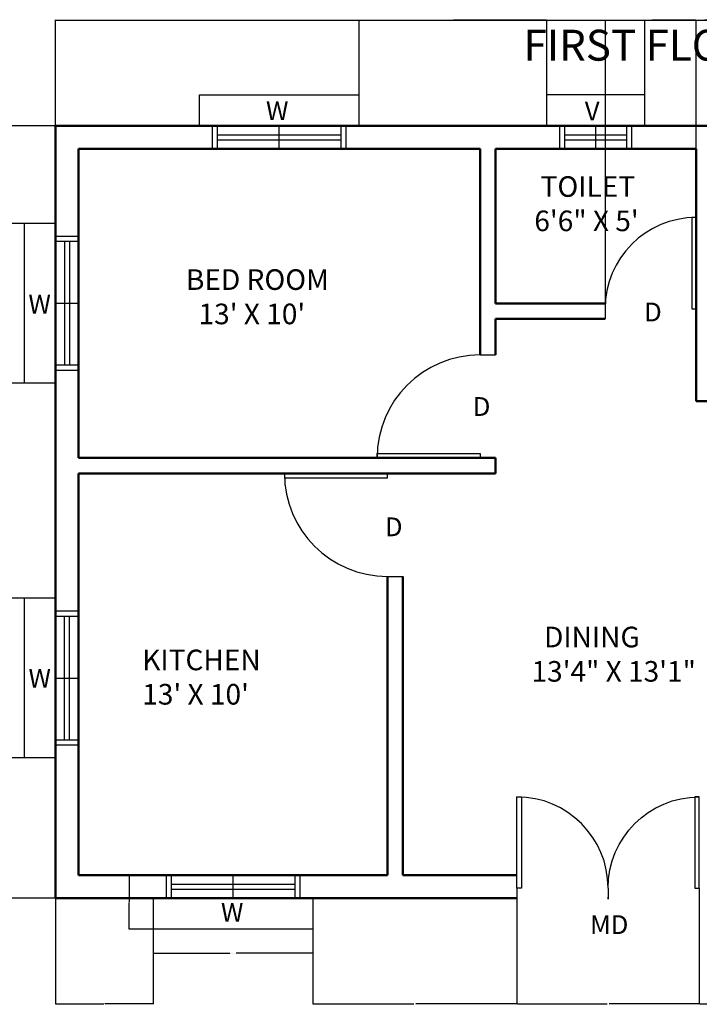
# Model space of a CAD drawing. Units: inches. Extents: x -73 to 1162, y -188 to 590.
# Tile 7 of 9: x 543 to 808, y -187 to 195. Entities that reach past the tile are written whole.
import ezdxf

# ---------------------------------------------------------------- set-up
doc = ezdxf.new("R2010")
doc.units = ezdxf.units.IN
doc.header["$MEASUREMENT"] = 0
for name, color, linetype, lineweight in [('A-ANNO-DIMS', 2, 'Continuous', 18), ('A-ANNO-TEXT', 7, 'Continuous', 25), ('A-AREA-IDEN', 2, 'Continuous', 25), ('A-DOOR', 3, 'Continuous', 25), ('A-GLAZ', 4, 'Continuous', 25), ('A-WALL', 7, 'Continuous', 50)]:
    doc.layers.add(name, color=color, linetype=linetype, lineweight=lineweight)
doc.styles.get("Standard").update_dxf_attribs({"font": 'arial.ttf'})
doc.dimstyles.get("Standard").update_dxf_attribs({"dimtxt": 0.18, "dimasz": 0.18, "dimexe": 0.18, "dimexo": 0.0625, "dimgap": 0.09, "dimtad": 0, "dimtih": 1, "dimtoh": 1, "dimdec": 1, "dimzin": 0, "dimdsep": 46, "dimlunit": 4, "dimtxsty": 'Standard', "dimcen": 0.09, "dimadec": 0, "dimazin": 0, "dimtfac": 1, "dimtdec": 1, "dimtofl": 0, "dimtmove": 0, "dimatfit": 3, "dimfxl": 1, "dimtolj": 1, "dimtzin": 0, "dimarcsym": 0})

# ---------------------------------------------------------------- blocks, each defined once
blk = doc.blocks.new('*U2')
for p, q in [((0, 0), (0, -6)), ((40, 0), (40, -6))]:
    blk.add_line(p, q)
blk.add_lwpolyline([(0, 0), (0, 40), (1.75, 40), (1.75, 0)], close=True)
blk.add_arc((0, 0), 40, 0, 90)
blk = doc.blocks.new('*U5')
for p, q in [((0, 0), (0, -100)), ((-900, 0), (-900, -100))]:
    blk.add_line(p, q)
blk.add_lwpolyline([(0, 0), (0, 900), (-43.75, 900), (-43.75, 0)], close=True)
blk.add_arc((0, 0), 900, 90, 180)
blk = doc.blocks.new('*U6')
for p, q in [((0, 0), (0, -6)), ((-40, 0), (-40, -6))]:
    blk.add_line(p, q)
blk.add_lwpolyline([(0, 0), (0, 40), (-1.75, 40), (-1.75, 0)], close=True)
blk.add_arc((0, 0), 40, 90, 180)
blk = doc.blocks.new('*U4')
for p, q in [((0, 0), (0, -100)), ((900, 0), (900, -100))]:
    blk.add_line(p, q)
blk.add_lwpolyline([(0, 0), (0, 900), (43.75, 900), (43.75, 0)], close=True)
blk.add_arc((0, 0), 900, 0, 90)
blk = doc.blocks.new('WIN-W')
for p, q in [((9, 57), (9, 62)), ((9, 62), (21, 62)), ((21, 62), (21, 0)), ((0, 57), (9, 57)), ((0, 5), (9, 5)), ((9, 5), (9, 0)), ((9, 0), (21, 0))]:
    blk.add_line(p, q)
blk = doc.blocks.new('VENT-V')
for p, q in [((0, 9), (0, 21)), ((38, 21), (0, 21)), ((38, 9), (38, 21)), ((5, 9), (0, 9)), ((5, 0), (5, 9)), ((33, 0), (33, 9)), ((33, 9), (38, 9))]:
    blk.add_line(p, q)
blk = doc.blocks.new('*D30')
at = {"layer": 'A-ANNO-DIMS', "color": 0, "lineweight": -2, "transparency": 16777216}
for p, q in [((595.31, -157.97), (595.31, -167.39)), ((657.31, -157.97), (657.31, -167.39)), ((595.49, -167.21), (625.04, -167.21)), ((657.13, -167.21), (627.58, -167.21))]:
    blk.add_line(p, q, dxfattribs=at)
at = {"layer": 'A-ANNO-DIMS', "color": 0, "transparency": 16777216}
for points in [[(595.49, -167.18), (595.49, -167.24), (595.31, -167.21)], [(657.13, -167.18), (657.13, -167.24), (657.31, -167.21)]]:
    blk.add_solid(points, dxfattribs=at)
at = {"layer": 'Defpoints', "color": 0, "transparency": 16777216}
for p in [(595.31, -157.91), (657.31, -157.91), (657.31, -167.21)]:
    blk.add_point(p, dxfattribs=at)
at = {"layer": 'A-ANNO-DIMS', "color": 0, "transparency": 16777216, "insert": (626.31, -167.21), "char_height": 0.18, "attachment_point": 5}
blk.add_mtext('\\A1;WINDOW W 62 TYP.', dxfattribs=at)
blk = doc.blocks.new('*D31')
at = {"layer": 'A-ANNO-DIMS', "color": 0, "lineweight": -2, "transparency": 16777216}
for p, q in [((595.24, -136.91), (585.83, -136.91)), ((586.01, -137.09), (586.01, -147.23)), ((586.01, -157.73), (586.01, -147.59)), ((595.24, -157.91), (585.83, -157.91))]:
    blk.add_line(p, q, dxfattribs=at)
at = {"layer": 'A-ANNO-DIMS', "color": 0, "transparency": 16777216}
for points in [[(585.98, -137.09), (586.04, -137.09), (586.01, -136.91)], [(585.98, -157.73), (586.04, -157.73), (586.01, -157.91)]]:
    blk.add_solid(points, dxfattribs=at)
at = {"layer": 'Defpoints', "color": 0, "transparency": 16777216}
for p in [(595.31, -136.91), (586.01, -157.91), (595.31, -157.91)]:
    blk.add_point(p, dxfattribs=at)
at = {"layer": 'A-ANNO-DIMS', "color": 0, "transparency": 16777216, "insert": (586.01, -147.41), "char_height": 0.18, "attachment_point": 5}
blk.add_mtext('\\A1;21 TYP.', dxfattribs=at)
blk = doc.blocks.new('*D100')
at = {"layer": 'A-ANNO-DIMS', "color": 0, "lineweight": -2, "transparency": 16777216}
for p, q in [((557.31, 154.15), (557.31, 195.27)), ((557.49, 195.09), (823.52, 195.09)), ((1090.13, 195.09), (824.1, 195.09)), ((1090.31, 154.15), (1090.31, 195.27))]:
    blk.add_line(p, q, dxfattribs=at)
at = {"layer": 'A-ANNO-DIMS', "color": 0, "transparency": 16777216}
for points in [[(557.49, 195.12), (557.49, 195.06), (557.31, 195.09)], [(1090.13, 195.12), (1090.13, 195.06), (1090.31, 195.09)]]:
    blk.add_solid(points, dxfattribs=at)
at = {"layer": 'Defpoints', "color": 0, "transparency": 16777216}
for p in [(1090.31, 195.09), (557.31, 154.09), (1090.31, 154.09)]:
    blk.add_point(p, dxfattribs=at)
at = {"layer": 'A-ANNO-DIMS', "color": 0, "transparency": 16777216, "insert": (823.81, 195.09), "char_height": 0.18, "attachment_point": 5}
blk.add_mtext('\\A1;533', dxfattribs=at)
blk = doc.blocks.new('*D101')
at = {"layer": 'A-ANNO-DIMS', "color": 0, "lineweight": -2, "transparency": 16777216}
for p, q in [((675.31, 166.15), (675.31, 195.27)), ((675.49, 195.09), (711.59, 195.09)), ((748.13, 195.09), (712.03, 195.09)), ((748.31, 166.15), (748.31, 195.27))]:
    blk.add_line(p, q, dxfattribs=at)
at = {"layer": 'A-ANNO-DIMS', "color": 0, "transparency": 16777216}
for points in [[(675.49, 195.12), (675.49, 195.06), (675.31, 195.09)], [(748.13, 195.12), (748.13, 195.06), (748.31, 195.09)]]:
    blk.add_solid(points, dxfattribs=at)
at = {"layer": 'Defpoints', "color": 0, "transparency": 16777216}
for p in [(748.31, 195.09), (675.31, 166.09), (748.31, 166.09)]:
    blk.add_point(p, dxfattribs=at)
at = {"layer": 'A-ANNO-DIMS', "color": 0, "transparency": 16777216, "insert": (711.81, 195.09), "char_height": 0.18, "attachment_point": 5}
blk.add_mtext('\\A1;73', dxfattribs=at)
blk = doc.blocks.new('*D102')
at = {"layer": 'A-ANNO-DIMS', "color": 0, "lineweight": -2, "transparency": 16777216}
for p, q in [((786.31, 166.15), (786.31, 195.27)), ((786.49, 195.09), (809.08, 195.09)), ((832.13, 195.09), (809.53, 195.09)), ((832.31, 166.15), (832.31, 195.27))]:
    blk.add_line(p, q, dxfattribs=at)
at = {"layer": 'A-ANNO-DIMS', "color": 0, "transparency": 16777216}
for points in [[(786.49, 195.12), (786.49, 195.06), (786.31, 195.09)], [(832.13, 195.12), (832.13, 195.06), (832.31, 195.09)]]:
    blk.add_solid(points, dxfattribs=at)
at = {"layer": 'Defpoints', "color": 0, "transparency": 16777216}
for p in [(832.31, 195.09), (786.31, 166.09), (832.31, 166.09)]:
    blk.add_point(p, dxfattribs=at)
at = {"layer": 'A-ANNO-DIMS', "color": 0, "transparency": 16777216, "insert": (809.31, 195.09), "char_height": 0.18, "attachment_point": 5}
blk.add_mtext('\\A1;46', dxfattribs=at)
blk = doc.blocks.new('*D104')
at = {"layer": 'A-ANNO-DIMS', "color": 0, "lineweight": -2, "transparency": 16777216}
for p, q in [((557.24, 154.09), (516.13, 154.09)), ((516.31, 153.91), (516.31, 4.27)), ((516.31, -145.73), (516.31, 3.91)), ((557.24, -145.91), (516.13, -145.91))]:
    blk.add_line(p, q, dxfattribs=at)
at = {"layer": 'A-ANNO-DIMS', "color": 0, "transparency": 16777216}
for points in [[(516.28, 153.91), (516.34, 153.91), (516.31, 154.09)], [(516.28, -145.73), (516.34, -145.73), (516.31, -145.91)]]:
    blk.add_solid(points, dxfattribs=at)
at = {"layer": 'Defpoints', "color": 0, "transparency": 16777216}
for p in [(557.31, 154.09), (516.31, -145.91), (557.31, -145.91)]:
    blk.add_point(p, dxfattribs=at)
at = {"layer": 'A-ANNO-DIMS', "color": 0, "transparency": 16777216, "insert": (516.31, 4.09), "char_height": 0.18, "attachment_point": 5}
blk.add_mtext('\\A1;300', dxfattribs=at)
blk = doc.blocks.new('*D105')
at = {"layer": 'A-ANNO-DIMS', "color": 0, "lineweight": -2, "transparency": 16777216}
for p, q in [((557.24, 154.09), (516.13, 154.09)), ((516.31, 153.91), (516.31, 135.27)), ((516.31, 116.27), (516.31, 134.91)), ((545.24, 116.09), (516.13, 116.09))]:
    blk.add_line(p, q, dxfattribs=at)
at = {"layer": 'A-ANNO-DIMS', "color": 0, "transparency": 16777216}
for points in [[(516.28, 153.91), (516.34, 153.91), (516.31, 154.09)], [(516.28, 116.27), (516.34, 116.27), (516.31, 116.09)]]:
    blk.add_solid(points, dxfattribs=at)
at = {"layer": 'Defpoints', "color": 0, "transparency": 16777216}
for p in [(557.31, 154.09), (516.31, 116.09), (545.31, 116.09)]:
    blk.add_point(p, dxfattribs=at)
at = {"layer": 'A-ANNO-DIMS', "color": 0, "transparency": 16777216, "insert": (516.31, 135.09), "char_height": 0.18, "attachment_point": 5}
blk.add_mtext('\\A1;38', dxfattribs=at)
blk = doc.blocks.new('*D106')
at = {"layer": 'A-ANNO-DIMS', "color": 0, "lineweight": -2, "transparency": 16777216}
for p, q in [((545.24, 54.09), (516.13, 54.09)), ((516.31, 53.91), (516.31, 12.52)), ((516.31, -29.23), (516.31, 12.16)), ((545.24, -29.41), (516.13, -29.41))]:
    blk.add_line(p, q, dxfattribs=at)
at = {"layer": 'A-ANNO-DIMS', "color": 0, "transparency": 16777216}
for points in [[(516.28, 53.91), (516.34, 53.91), (516.31, 54.09)], [(516.28, -29.23), (516.34, -29.23), (516.31, -29.41)]]:
    blk.add_solid(points, dxfattribs=at)
at = {"layer": 'Defpoints', "color": 0, "transparency": 16777216}
for p in [(545.31, 54.09), (516.31, -29.41), (545.31, -29.41)]:
    blk.add_point(p, dxfattribs=at)
at = {"layer": 'A-ANNO-DIMS', "color": 0, "transparency": 16777216, "insert": (516.31, 12.34), "char_height": 0.18, "attachment_point": 5}
blk.add_mtext('\\A1;83.5', dxfattribs=at)
blk = doc.blocks.new('*D107')
at = {"layer": 'A-ANNO-DIMS', "color": 0, "lineweight": -2, "transparency": 16777216}
for p, q in [((545.24, -91.41), (516.13, -91.41)), ((516.31, -91.59), (516.31, -118.48)), ((516.31, -145.73), (516.31, -118.84)), ((557.24, -145.91), (516.13, -145.91))]:
    blk.add_line(p, q, dxfattribs=at)
at = {"layer": 'A-ANNO-DIMS', "color": 0, "transparency": 16777216}
for points in [[(516.28, -91.59), (516.34, -91.59), (516.31, -91.41)], [(516.28, -145.73), (516.34, -145.73), (516.31, -145.91)]]:
    blk.add_solid(points, dxfattribs=at)
at = {"layer": 'Defpoints', "color": 0, "transparency": 16777216}
for p in [(545.31, -91.41), (516.31, -145.91), (557.31, -145.91)]:
    blk.add_point(p, dxfattribs=at)
at = {"layer": 'A-ANNO-DIMS', "color": 0, "transparency": 16777216, "insert": (516.31, -118.66), "char_height": 0.18, "attachment_point": 5}
blk.add_mtext('\\A1;54.5', dxfattribs=at)
blk = doc.blocks.new('*D108')
at = {"layer": 'A-ANNO-DIMS', "color": 0, "lineweight": -2, "transparency": 16777216}
for p, q in [((557.31, -145.97), (557.31, -187.09)), ((595.31, -157.97), (595.31, -187.09)), ((557.49, -186.91), (576.09, -186.91)), ((595.13, -186.91), (576.53, -186.91))]:
    blk.add_line(p, q, dxfattribs=at)
at = {"layer": 'A-ANNO-DIMS', "color": 0, "transparency": 16777216}
for points in [[(557.49, -186.88), (557.49, -186.94), (557.31, -186.91)], [(595.13, -186.88), (595.13, -186.94), (595.31, -186.91)]]:
    blk.add_solid(points, dxfattribs=at)
at = {"layer": 'Defpoints', "color": 0, "transparency": 16777216}
for p in [(557.31, -145.91), (595.31, -157.91), (595.31, -186.91)]:
    blk.add_point(p, dxfattribs=at)
at = {"layer": 'A-ANNO-DIMS', "color": 0, "transparency": 16777216, "insert": (576.31, -186.91), "char_height": 0.18, "attachment_point": 5}
blk.add_mtext('\\A1;38', dxfattribs=at)
blk = doc.blocks.new('*D109')
at = {"layer": 'A-ANNO-DIMS', "color": 0, "lineweight": -2, "transparency": 16777216}
for p, q in [((736.65, -145.97), (736.65, -187.09)), ((657.31, -157.97), (657.31, -187.09)), ((657.49, -186.91), (696.59, -186.91)), ((736.47, -186.91), (697.37, -186.91))]:
    blk.add_line(p, q, dxfattribs=at)
at = {"layer": 'A-ANNO-DIMS', "color": 0, "transparency": 16777216}
for points in [[(657.49, -186.88), (657.49, -186.94), (657.31, -186.91)], [(736.47, -186.88), (736.47, -186.94), (736.65, -186.91)]]:
    blk.add_solid(points, dxfattribs=at)
at = {"layer": 'Defpoints', "color": 0, "transparency": 16777216}
for p in [(736.65, -145.91), (657.31, -157.91), (736.65, -186.91)]:
    blk.add_point(p, dxfattribs=at)
at = {"layer": 'A-ANNO-DIMS', "color": 0, "transparency": 16777216, "insert": (696.98, -186.91), "char_height": 0.18, "attachment_point": 5}
blk.add_mtext('\\A1;79.35', dxfattribs=at)
blk = doc.blocks.new('*D110')
at = {"layer": 'A-ANNO-DIMS', "color": 0, "lineweight": -2, "transparency": 16777216}
for p, q in [((736.65, -145.97), (736.65, -187.09)), ((807.52, -145.97), (807.52, -187.09)), ((736.83, -186.91), (771.69, -186.91)), ((807.34, -186.91), (772.48, -186.91))]:
    blk.add_line(p, q, dxfattribs=at)
at = {"layer": 'A-ANNO-DIMS', "color": 0, "transparency": 16777216}
for points in [[(736.83, -186.88), (736.83, -186.94), (736.65, -186.91)], [(807.34, -186.88), (807.34, -186.94), (807.52, -186.91)]]:
    blk.add_solid(points, dxfattribs=at)
at = {"layer": 'Defpoints', "color": 0, "transparency": 16777216}
for p in [(736.65, -145.91), (807.52, -145.91), (807.52, -186.91)]:
    blk.add_point(p, dxfattribs=at)
at = {"layer": 'A-ANNO-DIMS', "color": 0, "transparency": 16777216, "insert": (772.09, -186.91), "char_height": 0.18, "attachment_point": 5}
blk.add_mtext('\\A1;70.87', dxfattribs=at)
blk = doc.blocks.new('*D111')
at = {"layer": 'A-ANNO-DIMS', "color": 0, "lineweight": -2, "transparency": 16777216}
for p, q in [((807.52, -145.97), (807.52, -187.09)), ((1090.31, -145.97), (1090.31, -187.09)), ((807.7, -186.91), (948.52, -186.91)), ((1090.13, -186.91), (949.31, -186.91))]:
    blk.add_line(p, q, dxfattribs=at)
at = {"layer": 'A-ANNO-DIMS', "color": 0, "transparency": 16777216}
for points in [[(807.7, -186.88), (807.7, -186.94), (807.52, -186.91)], [(1090.13, -186.88), (1090.13, -186.94), (1090.31, -186.91)]]:
    blk.add_solid(points, dxfattribs=at)
at = {"layer": 'Defpoints', "color": 0, "transparency": 16777216}
for p in [(807.52, -145.91), (1090.31, -145.91), (1090.31, -186.91)]:
    blk.add_point(p, dxfattribs=at)
at = {"layer": 'A-ANNO-DIMS', "color": 0, "transparency": 16777216, "insert": (948.91, -186.91), "char_height": 0.18, "attachment_point": 5}
blk.add_mtext('\\A1;282.8', dxfattribs=at)
blk = doc.blocks.new('*D117')
at = {"layer": 'A-ANNO-DIMS', "color": 0, "lineweight": -2, "transparency": 16777216}
for p, q in [((771.05, 85.15), (771.05, 195.27)), ((771.23, 195.09), (788.22, 195.09)), ((806.13, 195.09), (789.14, 195.09)), ((806.31, 85.15), (806.31, 195.27))]:
    blk.add_line(p, q, dxfattribs=at)
at = {"layer": 'A-ANNO-DIMS', "color": 0, "transparency": 16777216}
for points in [[(771.23, 195.12), (771.23, 195.06), (771.05, 195.09)], [(806.13, 195.12), (806.13, 195.06), (806.31, 195.09)]]:
    blk.add_solid(points, dxfattribs=at)
at = {"layer": 'Defpoints', "color": 0, "transparency": 16777216}
for p in [(806.31, 195.09), (771.05, 85.09), (806.31, 85.09)]:
    blk.add_point(p, dxfattribs=at)
at = {"layer": 'A-ANNO-DIMS', "color": 0, "transparency": 16777216, "insert": (788.68, 195.09), "char_height": 0.18, "attachment_point": 5}
blk.add_mtext('\\A1;35.256', dxfattribs=at)

msp = doc.modelspace()

# ---------------------------------------------------------------- linework, layer by layer
at = {"layer": 'A-GLAZ'}
for p, q in [((620.307, 145.0923), (620.307, 154.0923)), ((644.307, 145.0923), (644.307, 154.0923)), ((668.307, 145.0923), (668.307, 154.0923)), ((755.307, 145.0923), (755.307, 154.0923)), ((767.307, 145.0923), (767.307, 154.0923)), ((779.307, 145.0923), (779.307, 154.0923)), ((620.307, 150.5923), (668.307, 150.5923)), ((755.307, 150.5923), (779.307, 150.5923)), ((620.307, 148.5923), (668.307, 148.5923)), ((755.307, 148.5923), (779.307, 148.5923)), ((566.307, 109.0923), (557.307, 109.0923)), ((560.807, 109.0923), (560.807, 61.0923)), ((562.807, 109.0923), (562.807, 61.0923)), ((566.307, 85.0923), (557.307, 85.0923)), ((566.307, 61.0923), (557.307, 61.0923)), ((557.307, -36.4077), (566.307, -36.4077)), ((560.807, -84.4077), (560.807, -36.4077)), ((562.807, -84.4077), (562.807, -36.4077)), ((557.307, -60.4077), (566.307, -60.4077)), ((557.307, -84.4077), (566.307, -84.4077)), ((602.307, -136.9077), (602.307, -145.9077)), ((626.307, -136.9077), (626.307, -145.9077)), ((650.307, -136.9077), (650.307, -145.9077)), ((602.307, -140.4077), (650.307, -140.4077)), ((602.307, -142.4077), (650.307, -142.4077))]:
    msp.add_line(p, q, dxfattribs=at)
at = {"layer": 'A-WALL'}
for p, q in [((557.307, 154.0923), (728.307, 154.0923)), ((557.307, 154.0923), (557.307, 25.0923)), ((728.307, 154.0923), (812.307, 154.0923)), ((566.307, 145.0923), (722.307, 145.0923)), ((566.307, 145.0923), (566.307, 25.0923)), ((722.307, 145.0923), (722.307, 65.0923)), ((728.307, 145.0923), (728.307, 85.0923)), ((728.307, 145.0923), (806.307, 145.0923)), ((806.307, 47.0923), (806.307, 145.0923)), ((771.0508, 85.0923), (728.307, 85.0923)), ((806.307, 85.0923), (806.307, 79.0923)), ((728.307, 79.0923), (728.307, 65.0923)), ((770.8739, 79.0923), (728.307, 79.0923)), ((812.307, 47.0923), (806.307, 47.0923)), ((557.307, 25.0923), (557.307, -145.9077)), ((566.307, 25.0923), (728.307, 25.0923)), ((728.307, 25.0923), (728.307, 19.0923)), ((566.307, 19.0923), (686.307, 19.0923)), ((566.307, 19.0923), (566.307, -136.9077)), ((686.307, 19.0923), (728.307, 19.0923)), ((686.307, -136.9077), (686.307, -20.9077)), ((692.307, -136.9077), (692.307, -20.9077)), ((566.307, -136.9077), (686.307, -136.9077)), ((692.307, -136.9077), (736.6545, -136.9077)), ((557.307, -145.9077), (692.307, -145.9077)), ((692.307, -145.9077), (736.6545, -145.9077)), ((771.8682, -145.9077), (772.307, -145.9077)), ((771.8682, -145.9077), (772.307, -145.9077))]:
    msp.add_line(p, q, dxfattribs=at)

# ---------------------------------------------------------------- block references
at = {"layer": 'A-DOOR', "yscale": 0.0393700787401575, "zscale": 0.0393700787401575}
for name, p, xscale in [('*U5', (806.307, 83.0293), 0.0393700787401575), ('*U4', (736.6545, -141.9707), 0.0393700787401575), ('*U4', (807.5207, -141.9707), -0.0393700787401575)]:
    msp.add_blockref(name, p, dxfattribs=dict(at, xscale=xscale))
at = {"layer": 'A-DOOR', "rotation": 90}
for name, p in [('*U2', (722.307, 25.0923)), ('*U6', (686.307, 19.0923))]:
    msp.add_blockref(name, p, dxfattribs=at)
at = {"layer": 'A-GLAZ'}
for p, rotation in [((675.3075, 145.0923), 90.00000000000007), ((566.307, 116.0927), 180), ((566.307, -29.4073), 180), ((595.3066, -136.9077), 270.0000000000001)]:
    msp.add_blockref('WIN-W', p, dxfattribs=dict(at, rotation=rotation))
msp.add_blockref('VENT-V', (748.307, 145.0919), dxfattribs=at)

# ---------------------------------------------------------------- texts
at = {"layer": 'A-ANNO-TEXT'}
for s, height, p in [('W', 7.2829, (639.1433, 156.262)), ('V', 7.2829, (763.0334, 156.1282)), ('W', 7.2829, (546.8381, 81.1694)), ('D', 7.2829, (786.089, 78.1092)), ('D', 7.2829, (719.5144, 41.4112)), ('D', 7.2829, (685.3668, -5.3162)), ('W', 7.2829, (546.8697, -64.0987)), ('W', 7.2829, (621.6447, -155.0471)), ('MD', 7.28289, (765.0631, -159.7922))]:
    msp.add_text(s, height=height, dxfattribs=at).set_placement(p)
at = {"layer": 'A-ANNO-TEXT', "insert": (739.1941, 191.3681), "char_height": 12, "attachment_point": 1}
msp.add_mtext_dynamic_manual_height_columns('FIRST FLOOR PLAN', width=198.609453, gutter_width=1, heights=[0], dxfattribs=at)
at = {"layer": 'A-AREA-IDEN', "char_height": 8, "attachment_point": 1}
for s, insert in [(' TOILET\\P6\'6" X 5\'', (743.4101, 134.486)), ("BED ROOM\\P  13' X 10'", (608.0547, 98.3426)), ('  DINING\\P13\'4" X 13\'1"', (742.3067, -40.4541)), ("KITCHEN\\P13' X 10'", (591.0725, -49.3583))]:
    msp.add_mtext_dynamic_manual_height_columns(s, width=71.534965, gutter_width=1, heights=[0], dxfattribs=dict(at, insert=insert))

# ---------------------------------------------------------------- dimensions: what is measured, and where the dimension line sits
at = {"layer": 'A-ANNO-DIMS'}
for base, p1, p2, override, picture, middle in [((1090.307, 195.0923), (557.307, 154.0923), (1090.307, 154.0923), {"dimdec": 0, "dimlfac": 1, "dimrnd": 0, "dimzin": 0, "dimdsep": 46, "dimlunit": 2}, '*D100', (823.807, 195.0923)), ((748.307, 195.0923), (675.307, 166.0923), (748.307, 166.0923), {"dimdec": 0, "dimlfac": 1, "dimrnd": 0, "dimzin": 0, "dimdsep": 46, "dimlunit": 2}, '*D101', (711.807, 195.0923)), ((806.307, 195.0923), (771.0508, 85.0923), (806.307, 85.0923), {"dimdec": 3, "dimlfac": 1, "dimrnd": 0, "dimzin": 0, "dimdsep": 46, "dimlunit": 2}, '*D117', (788.6789, 195.0923)), ((832.307, 195.0923), (786.307, 166.0923), (832.307, 166.0923), {"dimdec": 0, "dimlfac": 1, "dimrnd": 0, "dimzin": 0, "dimdsep": 46, "dimlunit": 2}, '*D102', (809.307, 195.0923)), ((595.307, -186.9077), (557.307, -145.9077), (595.307, -157.9077), {"dimdec": 0, "dimlfac": 1, "dimrnd": 0, "dimzin": 0, "dimdsep": 46, "dimlunit": 2}, '*D108', (576.307, -186.9077)), ((736.6545, -186.9077), (657.307, -157.9077), (736.6545, -145.9077), {"dimdec": 2, "dimlfac": 1, "dimrnd": 0, "dimzin": 0, "dimdsep": 46, "dimlunit": 2}, '*D109', (696.9808, -186.9077)), ((807.5207, -186.9077), (736.6545, -145.9077), (807.5207, -145.9077), {"dimdec": 2, "dimlfac": 1, "dimrnd": 0, "dimzin": 0, "dimdsep": 46, "dimlunit": 2}, '*D110', (772.0876, -186.9077)), ((1090.307, -186.9077), (807.5207, -145.9077), (1090.307, -145.9077), {"dimdec": 1, "dimlfac": 1, "dimrnd": 0, "dimzin": 0, "dimdsep": 46, "dimlunit": 2}, '*D111', (948.9139, -186.9077))]:
    dim = msp.add_linear_dim(base=base, p1=p1, p2=p2, dimstyle='Standard', override=override, dxfattribs=at)
    dim.commit()
    dim.dimension.update_dxf_attribs({"geometry": picture, "text_midpoint": middle})
for base, p1, p2, override, picture, middle in [((516.307, -145.9077), (557.307, 154.0923), (557.307, -145.9077), {"dimdec": 0, "dimlfac": 1, "dimrnd": 0, "dimzin": 0, "dimdsep": 46, "dimlunit": 2}, '*D104', (516.307, 4.0923)), ((516.307, 116.0923), (557.307, 154.0923), (545.307, 116.0923), {"dimdec": 0, "dimlfac": 1, "dimrnd": 0, "dimzin": 0, "dimdsep": 46, "dimlunit": 2}, '*D105', (516.307, 135.0923)), ((516.307, -29.4077), (545.307, 54.0923), (545.307, -29.4077), {"dimdec": 1, "dimlfac": 1, "dimrnd": 0, "dimzin": 0, "dimdsep": 46, "dimlunit": 2}, '*D106', (516.307, 12.3423)), ((516.307, -145.9077), (545.307, -91.4077), (557.307, -145.9077), {"dimdec": 1, "dimlfac": 1, "dimrnd": 0, "dimzin": 0, "dimdsep": 46, "dimlunit": 2}, '*D107', (516.307, -118.6577))]:
    dim = msp.add_linear_dim(base=base, p1=p1, p2=p2, angle=90, dimstyle='Standard', override=override, dxfattribs=at)
    dim.commit()
    dim.dimension.update_dxf_attribs({"geometry": picture, "text_midpoint": middle})
for base, p1, p2, angle, text, picture, middle in [((586.007, -157.9077), (595.307, -136.9077), (595.307, -157.9077), 270, '<> TYP.', '*D31', (586.007, -147.4077)), ((657.307, -167.2077), (595.307, -157.9077), (657.307, -157.9077), 0, 'WINDOW W <> TYP.', '*D30', (626.307, -167.2077))]:
    dim = msp.add_linear_dim(base=base, p1=p1, p2=p2, angle=angle, text=text, dimstyle='Standard', override={"dimdec": 0, "dimrnd": 0, "dimzin": 0, "dimlunit": 2}, dxfattribs=at)
    dim.commit()
    dim.dimension.update_dxf_attribs({"geometry": picture, "text_midpoint": middle})

doc.saveas('drawing.dxf')
